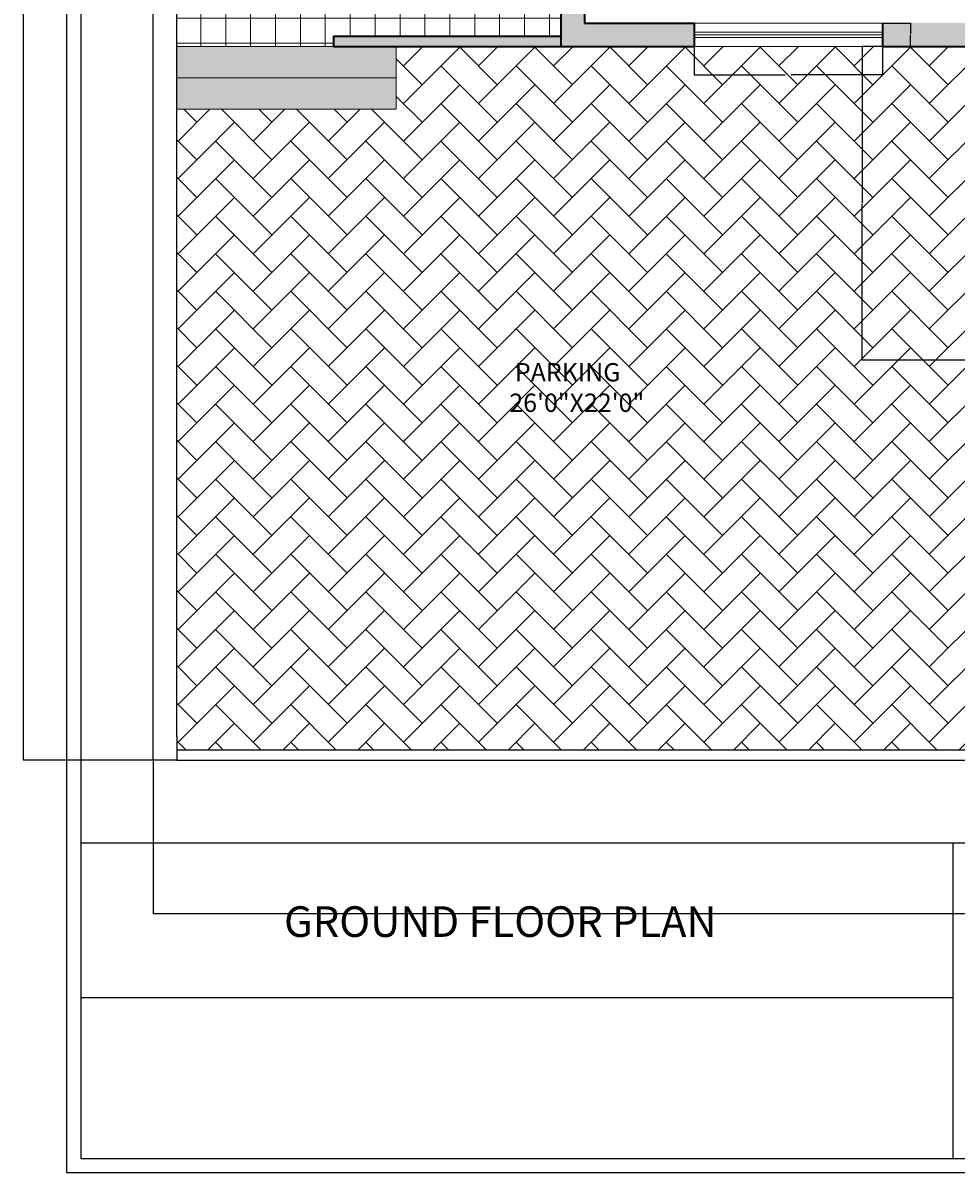
# Model space of a CAD drawing. Units: inches. Extents: x 84 to 1044, y -280 to 906.
# Tile 1 of 105: x 84 to 441, y -280 to 160. Entities that reach past the tile are written whole.
import ezdxf

# ---------------------------------------------------------------- set-up
doc = ezdxf.new("R2010")
doc.units = ezdxf.units.IN
for name, color, linetype, lineweight in [('A-ANNO-DIMS', 2, 'Continuous', 18), ('A-ANNO-TTLB', 7, 'Continuous', 25), ('A-AREA-IDEN', 7, 'Continuous', 13), ('A-STAIRCASE', 144, 'Continuous', 18), ('C-PROP', 7, 'Continuous', 25), ('L-HRDS', 32, 'Continuous', 18), ('WALL', 250, 'Continuous', 35), ('WINDOW', 160, 'Continuous', 13)]:
    doc.layers.add(name, color=color, linetype=linetype, lineweight=lineweight)
for name, color, linetype, lineweight, true_color in [('A-FLOR-PATT', 251, 'Continuous', 9, 0x705861), ('A-FLOR-STRS-PATT', 35, 'Continuous', 9, 0x947764), ('A-WALL-PATT', 251, 'Continuous', 9, 0x636466), ('L-PRKG-PATT', 35, 'Continuous', 9, 0x947764)]:
    doc.layers.add(name, color=color, linetype=linetype, lineweight=lineweight, true_color=true_color)
doc.styles.add('1-100DIM', font='txt', dxfattribs={"height": 0.3})
doc.styles.get("Standard").update_dxf_attribs({"font": 'arial.ttf'})
doc.dimstyles.get("Standard").update_dxf_attribs({"dimtxt": 0.18, "dimasz": 0.18, "dimexe": 0.18, "dimexo": 0.0625, "dimgap": 0.09, "dimtad": 0, "dimtih": 1, "dimtoh": 1, "dimdec": 4, "dimzin": 0, "dimdsep": 46, "dimtxsty": 'Standard', "dimcen": 0.09, "dimadec": 0, "dimazin": 0, "dimtfac": 1, "dimtdec": 4, "dimtofl": 0, "dimtmove": 0, "dimatfit": 3, "dimfxl": 1, "dimtolj": 1, "dimtzin": 0, "dimarcsym": 0})

# ---------------------------------------------------------------- blocks, each defined once
blk = doc.blocks.new('WIN-72IN')
for p, q in [((72, 9), (0, 9)), ((72, 5.5), (0, 5.5)), ((72, 4.5), (0, 4.5)), ((72, 3.5), (0, 3.5)), ((0, 0), (72, 0))]:
    blk.add_line(p, q)
blk = doc.blocks.new('*D34')
at = {"layer": 'A-ANNO-DIMS', "color": 0, "lineweight": -2, "transparency": 16777216}
for p, q in [((341.13, 151.06), (341.13, 140.14)), ((413.13, 151.06), (413.13, 140.14)), ((341.31, 140.32), (376.01, 140.32)), ((412.95, 140.32), (378.24, 140.32))]:
    blk.add_line(p, q, dxfattribs=at)
at = {"layer": 'A-ANNO-DIMS', "color": 0, "transparency": 16777216}
for points in [[(341.31, 140.35), (341.31, 140.29), (341.13, 140.32)], [(412.95, 140.35), (412.95, 140.29), (413.13, 140.32)]]:
    blk.add_solid(points, dxfattribs=at)
at = {"layer": 'Defpoints', "color": 0, "transparency": 16777216}
for p in [(341.13, 151.12), (413.13, 151.12), (413.13, 140.32)]:
    blk.add_point(p, dxfattribs=at)
at = {"layer": 'A-ANNO-DIMS', "color": 0, "transparency": 16777216, "insert": (377.13, 140.32), "char_height": 0.18, "attachment_point": 5}
blk.add_mtext('\\A1;WINDOW 72 TYP.', dxfattribs=at)
blk = doc.blocks.new('*D35')
at = {"layer": 'A-ANNO-DIMS', "color": 0, "lineweight": -2, "transparency": 16777216}
for p, q in [((413.19, 160.12), (424.11, 160.12)), ((423.93, 159.94), (423.93, 155.8)), ((423.93, 151.3), (423.93, 155.44)), ((413.19, 151.12), (424.11, 151.12))]:
    blk.add_line(p, q, dxfattribs=at)
at = {"layer": 'A-ANNO-DIMS', "color": 0, "transparency": 16777216}
for points in [[(423.9, 159.94), (423.96, 159.94), (423.93, 160.12)], [(423.9, 151.3), (423.96, 151.3), (423.93, 151.12)]]:
    blk.add_solid(points, dxfattribs=at)
at = {"layer": 'Defpoints', "color": 0, "transparency": 16777216}
for p in [(413.13, 160.12), (423.93, 160.12), (413.13, 151.12)]:
    blk.add_point(p, dxfattribs=at)
at = {"layer": 'A-ANNO-DIMS', "color": 0, "transparency": 16777216, "insert": (423.93, 155.62), "char_height": 0.18, "attachment_point": 5}
blk.add_mtext('\\A1;9 TYP.', dxfattribs=at)
blk = doc.blocks.new('*D60')
at = {"layer": 'A-ANNO-DIMS', "color": 0, "lineweight": -2, "transparency": 16777216}
for p, q in [((134.18, -121.94), (134.18, -180.64)), ((992.07, -121.94), (992.07, -180.64)), ((134.36, -180.46), (562.73, -180.46)), ((991.89, -180.46), (563.52, -180.46))]:
    blk.add_line(p, q, dxfattribs=at)
at = {"layer": 'A-ANNO-DIMS', "color": 0, "transparency": 16777216}
for points in [[(134.36, -180.43), (134.36, -180.49), (134.18, -180.46)], [(991.89, -180.43), (991.89, -180.49), (992.07, -180.46)]]:
    blk.add_solid(points, dxfattribs=at)
at = {"layer": 'Defpoints', "color": 0, "transparency": 16777216}
for p in [(134.18, -121.88), (992.07, -121.88), (992.07, -180.46)]:
    blk.add_point(p, dxfattribs=at)
at = {"layer": 'A-ANNO-DIMS', "color": 0, "transparency": 16777216, "insert": (563.13, -180.46), "char_height": 0.18, "attachment_point": 5}
blk.add_mtext('\\A1;857.9', dxfattribs=at)
blk = doc.blocks.new('*D61')
at = {"layer": 'A-ANNO-DIMS', "color": 0, "lineweight": -2, "transparency": 16777216}
for p, q in [((134.12, 856.12), (84.4, 856.12)), ((84.58, 855.94), (84.58, 367.3)), ((84.58, -121.7), (84.58, 366.94)), ((134.12, -121.88), (84.4, -121.88))]:
    blk.add_line(p, q, dxfattribs=at)
at = {"layer": 'A-ANNO-DIMS', "color": 0, "transparency": 16777216}
for points in [[(84.55, 855.94), (84.61, 855.94), (84.58, 856.12)], [(84.55, -121.7), (84.61, -121.7), (84.58, -121.88)]]:
    blk.add_solid(points, dxfattribs=at)
at = {"layer": 'Defpoints', "color": 0, "transparency": 16777216}
for p in [(84.58, 856.12), (134.18, 856.12), (134.18, -121.88)]:
    blk.add_point(p, dxfattribs=at)
at = {"layer": 'A-ANNO-DIMS', "color": 0, "transparency": 16777216, "insert": (84.58, 367.12), "char_height": 0.18, "attachment_point": 5}
blk.add_mtext('\\A1;978', dxfattribs=at)
blk = doc.blocks.new('*D80')
at = {"layer": 'A-ANNO-DIMS', "color": 0, "lineweight": -2, "transparency": 16777216}
for p, q in [((455.01, 151.12), (405.29, 151.12)), ((405.47, 150.94), (405.47, 91.3)), ((405.47, 31.3), (405.47, 90.94)), ((455.01, 31.12), (405.29, 31.12))]:
    blk.add_line(p, q, dxfattribs=at)
at = {"layer": 'A-ANNO-DIMS', "color": 0, "transparency": 16777216}
for points in [[(405.44, 150.94), (405.5, 150.94), (405.47, 151.12)], [(405.44, 31.3), (405.5, 31.3), (405.47, 31.12)]]:
    blk.add_solid(points, dxfattribs=at)
at = {"layer": 'Defpoints', "color": 0, "transparency": 16777216}
for p in [(405.47, 151.12), (455.07, 151.12), (455.07, 31.12)]:
    blk.add_point(p, dxfattribs=at)
at = {"layer": 'A-ANNO-DIMS', "color": 0, "transparency": 16777216, "insert": (405.47, 91.12), "char_height": 0.18, "attachment_point": 5}
blk.add_mtext('\\A1;120', dxfattribs=at)

msp = doc.modelspace()

# ---------------------------------------------------------------- hatches: boundary and pattern name
at = {"layer": 'A-FLOR-PATT', "transparency": 33554597}
h = msp.add_hatch(dxfattribs=at)
h.set_pattern_fill('ANSI37', color=256, scale=3, angle=45)
h.paths.add_polyline_path([(290.179, 211.12), (299.179, 211.12), (299.179, 247.12), (203.179, 247.12), (143.179, 247.12), (143.179, 151.12), (203.179, 151.12), (203.179, 155.12), (290.179, 155.12)])
at = {"layer": 'A-FLOR-STRS-PATT', "transparency": 33554567}
h = msp.add_hatch(color=256, dxfattribs=at)
h.dxf.hatch_style = 1
h.paths.add_polyline_path([(650.074, 91.12), (638.074, 91.12), (638.074, 67.12), (455.074, 67.12), (455.074, 55.12), (650.074, 55.12)], flags=17)
h.paths.add_polyline_path([(662.074, 91.12), (650.074, 91.12), (650.074, 55.12), (455.074, 55.12), (455.074, 43.12), (662.074, 43.12)])
h.paths.add_polyline_path([(674.074, 91.12), (671.074, 91.12), (662.074, 91.12), (662.074, 43.12), (455.074, 43.12), (455.074, 31.12), (674.074, 31.12)])
h.paths.add_polyline_path([(227.179, 151.12), (203.179, 151.12), (143.179, 151.12), (143.179, 139.12), (227.179, 139.12)])
h.paths.add_polyline_path([(227.179, 139.12), (143.179, 139.12), (143.179, 127.12), (227.179, 127.12)])
h.paths.add_polyline_path([(203.179, 271.12), (143.179, 271.12), (143.179, 259.12), (203.179, 259.12)])
h.paths.add_polyline_path([(203.179, 259.12), (143.179, 259.12), (143.179, 247.12), (203.179, 247.12)])
h.paths.add_polyline_path([(203.179, 769.12), (143.179, 769.12), (143.179, 757.12), (203.179, 757.12)])
h.paths.add_polyline_path([(203.179, 757.12), (143.179, 757.12), (143.179, 745.12), (203.179, 745.12)])
h.paths.add_polyline_path([(434.074, 847.12), (422.074, 847.12), (422.074, 769.12), (434.074, 769.12)])
h.paths.add_polyline_path([(422.074, 847.12), (410.074, 847.12), (410.074, 769.12), (422.074, 769.12)])
at = {"layer": 'A-WALL-PATT', "transparency": 33554597}
h = msp.add_hatch(color=256, dxfattribs=at)
h.dxf.hatch_style = 1
h.paths.add_polyline_path([(671.074, 100.12), (647.074, 100.12), (647.074, 160.12), (641.074, 160.12), (620.824, 160.12), (620.824, 151.12), (638.074, 151.12), (638.074, 91.12), (671.074, 91.12)])
h.paths.add_polyline_path([(791.074, 100.12), (743.074, 100.12), (743.074, 91.12), (791.074, 91.12)])
h.paths.add_polyline_path([(896.074, 346.12), (887.074, 346.12), (887.074, 334.12), (870.955, 334.12), (833.074, 334.12), (804.574, 334.12), (804.574, 328.12), (887.074, 328.12), (887.074, 100.12), (863.074, 100.12), (863.074, 91.12), (896.074, 91.12)])
h.paths.add_polyline_path([(507.574, 154.729), (507.574, 160.12), (464.074, 160.12), (464.074, 247.12), (641.074, 247.12), (641.074, 208.12), (647.074, 208.12), (647.074, 328.12), (659.074, 328.12), (659.074, 334.12), (617.074, 334.12), (617.074, 328.12), (641.074, 328.12), (641.074, 256.12), (545.074, 256.12), (545.074, 328.12), (569.074, 328.12), (569.074, 334.12), (518.074, 334.12), (518.074, 325.12), (536.074, 325.12), (536.074, 256.12), (464.074, 256.12), (464.074, 325.12), (482.074, 325.12), (482.074, 334.12), (455.074, 334.12), (455.074, 160.12), (413.127, 160.12), (413.127, 151.12), (455.074, 151.12), (455.074, 91.12), (464.074, 91.12), (464.074, 151.12), (507.574, 151.12)])
h.paths.add_polyline_path([(572.824, 160.12), (555.574, 160.12), (555.574, 151.12), (572.824, 151.12)], flags=17)
h.paths.add_polyline_path([(341.127, 160.12), (299.179, 160.12), (299.179, 211.12), (294.179, 211.12), (290.179, 211.12), (290.179, 151.12), (341.127, 151.12)])
h.paths.add_polyline_path([(299.179, 256.12), (212.179, 256.12), (212.179, 274.12), (203.179, 274.12), (203.179, 247.12), (299.179, 247.12)])
h.paths.add_polyline_path([(212.179, 514.12), (398.074, 514.12), (398.074, 519.12), (398.074, 520.12), (212.179, 520.12), (212.179, 574.12), (203.179, 574.12), (203.179, 310.12), (212.179, 310.12), (212.179, 328.12), (290.179, 328.12), (290.179, 292.12), (299.179, 292.12), (299.179, 328.12), (332.179, 328.12), (332.179, 334.12), (212.179, 334.12)])
h.paths.add_polyline_path([(287.127, 709.12), (203.179, 709.12), (203.179, 646.12), (212.179, 646.12), (212.179, 700.12), (287.127, 700.12)])
h.paths.add_polyline_path([(470.074, 709.12), (359.127, 709.12), (359.127, 700.12), (434.074, 700.12), (434.074, 574.12), (440.074, 574.12), (440.074, 622.12), (464.074, 622.12), (464.074, 628.12), (440.074, 628.12), (440.074, 700.12), (470.074, 700.12)])
h.paths.add_polyline_path([(572.074, 709.12), (506.074, 709.12), (506.074, 700.12), (536.074, 700.12), (536.074, 628.12), (494.074, 628.12), (494.074, 622.12), (536.074, 622.12), (536.074, 520.12), (440.074, 520.12), (440.074, 544.12), (434.074, 544.12), (434.074, 514.12), (644.074, 514.12), (644.074, 519.12), (644.074, 544.12), (638.074, 544.12), (638.074, 520.12), (542.074, 520.12), (542.074, 622.12), (584.074, 622.12), (584.074, 628.12), (542.074, 628.12), (542.074, 700.12), (572.074, 700.12)])
h.paths.add_polyline_path([(698.074, 709.12), (608.074, 709.12), (608.074, 700.12), (638.074, 700.12), (638.074, 628.12), (614.074, 628.12), (614.074, 622.12), (638.074, 622.12), (638.074, 574.12), (644.074, 574.12), (644.074, 700.12), (698.074, 700.12)])
h.paths.add_polyline_path([(833.074, 709.12), (770.074, 709.12), (770.074, 700.12), (824.074, 700.12), (824.074, 646.12), (833.074, 646.12)])
h.paths.add_polyline_path([(833.074, 574.12), (824.074, 574.12), (824.074, 520.12), (791.244, 520.12), (712.904, 520.12), (680.074, 520.12), (680.074, 514.12), (695.074, 514.12), (695.074, 491.62), (704.074, 491.62), (704.074, 511.12), (833.074, 511.12)])
h.paths.add_polyline_path([(704.074, 419.62), (695.074, 419.62), (695.074, 370.12), (704.074, 370.12)])
h.paths.add_polyline_path([(896.074, 400.12), (833.074, 400.12), (833.074, 364.12), (839.074, 364.12), (839.074, 394.12), (887.074, 394.12), (887.074, 382.12), (896.074, 382.12)])
h.paths.add_polyline_path([(732.574, 334.12), (695.074, 334.12), (695.074, 328.12), (732.574, 328.12)])
h = msp.add_hatch(color=256, dxfattribs=at)
h.dxf.hatch_style = 1
h.paths.add_polyline_path([(290.179, 155.12), (203.179, 155.12), (203.179, 151.12), (290.179, 151.12)])
at = {"layer": 'L-PRKG-PATT', "transparency": 33554567}
h = msp.add_hatch(dxfattribs=at)
h.set_pattern_fill('AR-HBONE', color=256, scale=0.1)
h.paths.add_polyline_path([(455.074, 31.12), (455.074, 91.12), (455.074, 151.12), (413.127, 151.12), (341.127, 151.12), (290.179, 151.12), (227.179, 151.12), (227.179, 127.12), (143.179, 127.12), (143.179, -112.88), (143.179, -117.88), (455.074, -117.88)])

# ---------------------------------------------------------------- linework, layer by layer
at = {"layer": 'A-ANNO-TTLB'}
for p, q in [((106.576, -153.519), (1021.832, -153.519)), ((440.274, -274.288), (440.274, -153.519)), ((106.576, -212.591), (440.274, -212.591))]:
    msp.add_line(p, q, dxfattribs=at)
for points in [[(101.1, 905.916), (1027.308, 905.916), (1027.308, -279.764), (101.1, -279.764)], [(106.576, 900.439), (1021.832, 900.439), (1021.832, -274.288), (106.576, -274.288)]]:
    msp.add_lwpolyline(points, close=True, dxfattribs=at)
at = {"layer": 'A-STAIRCASE'}
for p, q in [((143.179, 247.12), (143.179, 127.12)), ((227.179, 127.12), (227.179, 151.12)), ((227.179, 139.12), (143.179, 139.12)), ((227.179, 127.12), (143.179, 127.12))]:
    msp.add_line(p, q, dxfattribs=at)
at = {"layer": 'C-PROP'}
for p, q in [((143.179, -112.88), (143.179, -121.88)), ((143.179, -117.88), (455.074, -117.88)), ((143.179, -121.88), (455.074, -121.88))]:
    msp.add_line(p, q, dxfattribs=at)
for points in [[(143.179, -121.88), (134.179, -121.88), (134.179, 856.12), (992.074, 856.12), (992.074, -121.88), (624.574, -121.88)], [(143.179, -112.88), (143.179, 847.12), (983.074, 847.12), (983.074, -112.88), (624.574, -112.88)]]:
    msp.add_lwpolyline(points, dxfattribs=at)
at = {"layer": 'L-HRDS'}
msp.add_line((203.179, 151.12), (143.179, 151.12), dxfattribs=at)
at = {"layer": 'WALL'}
for p, q in [((290.179, 211.12), (290.179, 151.12)), ((299.179, 211.12), (299.179, 160.12)), ((299.179, 160.12), (341.127, 160.12)), ((341.127, 160.12), (341.127, 151.12)), ((413.127, 160.12), (413.127, 151.12)), ((203.179, 155.12), (203.179, 151.12)), ((290.179, 151.12), (341.127, 151.12)), ((413.127, 151.12), (455.074, 151.12))]:
    msp.add_line(p, q, dxfattribs=at)
for points in [[(203.179, 155.12), (290.179, 155.12)], [(203.179, 151.12), (290.179, 151.12)]]:
    msp.add_lwpolyline(points, dxfattribs=at)

# ---------------------------------------------------------------- block references
at = {"layer": 'WINDOW'}
msp.add_blockref('WIN-72IN', (341.123, 151.12), dxfattribs=at)

# ---------------------------------------------------------------- texts
at = {"layer": 'A-ANNO-TTLB', "insert": (184.229, -177.755), "char_height": 11.70049, "attachment_point": 1, "style": '1-100DIM'}
msp.add_mtext_dynamic_manual_height_columns('{\\f@Malgun Gothic|b0|i0|c0|p34;GROUND FLOOR PLAN  }', width=278.81784, gutter_width=24.488, heights=[0], dxfattribs=at)
at = {"layer": 'A-AREA-IDEN', "insert": (270.429, 30.026), "char_height": 7, "attachment_point": 1, "style": '1-100DIM'}
msp.add_mtext_dynamic_manual_height_columns('{\\f@Malgun Gothic|b0|i0|c0|p34; PARKING\\P26\'0"X22\'0"}', width=42.68803, gutter_width=15.851, heights=[0], dxfattribs=at)

# ---------------------------------------------------------------- dimensions: what is measured, and where the dimension line sits
at = {"layer": 'A-ANNO-DIMS'}
for base, p1, p2, picture, middle in [((84.579, 856.12), (134.179, -121.88), (134.179, 856.12), '*D61', (84.579, 367.12)), ((405.474, 151.12), (455.074, 31.12), (455.074, 151.12), '*D80', (405.474, 91.12))]:
    dim = msp.add_linear_dim(base=base, p1=p1, p2=p2, angle=90, dimstyle='Standard', override={"dimdec": 0, "dimlfac": 1, "dimrnd": 0, "dimzin": 0, "dimdsep": 46, "dimlunit": 2}, dxfattribs=at)
    dim.commit()
    dim.dimension.update_dxf_attribs({"geometry": picture, "text_midpoint": middle})
dim = msp.add_linear_dim(base=(423.927, 160.12), p1=(413.127, 151.12), p2=(413.127, 160.12), angle=90, text='<> TYP.', dimstyle='Standard', override={"dimdec": 0, "dimlfac": 1, "dimrnd": 0, "dimzin": 0, "dimdsep": 46, "dimlunit": 2}, dxfattribs=at)
dim.commit()
dim.dimension.update_dxf_attribs({"geometry": '*D35', "text_midpoint": (423.927, 155.62)})
dim = msp.add_linear_dim(base=(413.127, 140.32), p1=(341.127, 151.12), p2=(413.127, 151.12), text='WINDOW <> TYP.', dimstyle='Standard', override={"dimdec": 0, "dimlfac": 1, "dimrnd": 0, "dimzin": 0, "dimdsep": 46, "dimlunit": 2}, dxfattribs=at)
dim.commit()
dim.dimension.update_dxf_attribs({"geometry": '*D34', "text_midpoint": (377.127, 140.32)})
dim = msp.add_linear_dim(base=(992.074, -180.46), p1=(134.179, -121.88), p2=(992.074, -121.88), dimstyle='Standard', override={"dimdec": 1, "dimlfac": 1, "dimrnd": 0, "dimzin": 0, "dimdsep": 46, "dimlunit": 2}, dxfattribs=at)
dim.commit()
dim.dimension.update_dxf_attribs({"geometry": '*D60', "text_midpoint": (563.127, -180.46)})

doc.saveas('drawing.dxf')
